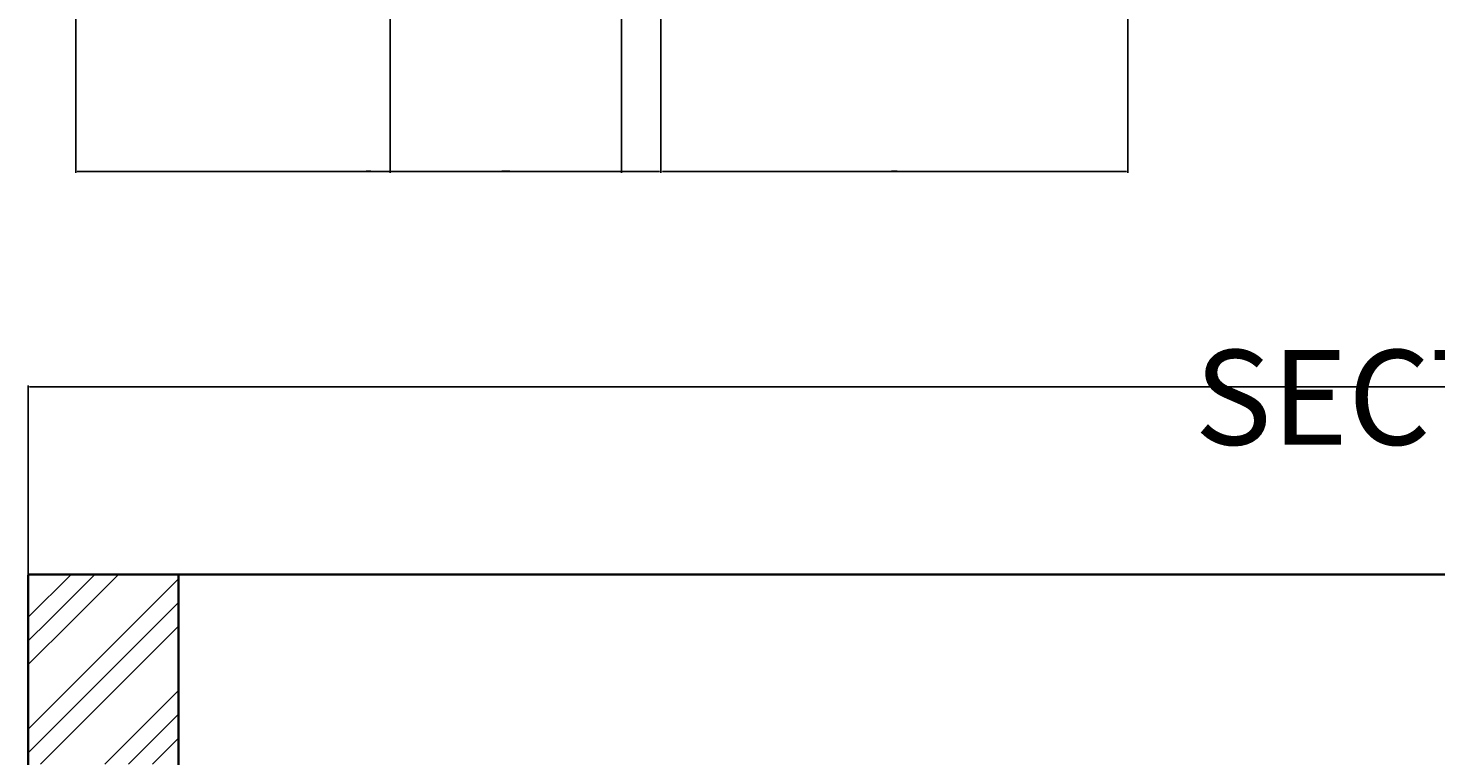
# Model space of a CAD drawing. Units: inches. Extents: x -128 to 854, y -395 to 398.
# Tile 12 of 61: x -56 to 122, y -201 to -109. Entities that reach past the tile are written whole.
import ezdxf

# ---------------------------------------------------------------- set-up
doc = ezdxf.new("R2010")
doc.units = ezdxf.units.IN
doc.header["$MEASUREMENT"] = 0
for name, color, linetype, lineweight in [('A-ANNO-DIMS', 2, 'Continuous', 18), ('A-ANNO-TITL', 7, 'Continuous', 25), ('A-SECT', 220, 'Continuous', 35), ('A-SECT-PATT', 8, 'Continuous', 13)]:
    doc.layers.add(name, color=color, linetype=linetype, lineweight=lineweight)
doc.styles.get("Standard").update_dxf_attribs({"font": 'arial.ttf'})
doc.dimstyles.get("Standard").update_dxf_attribs({"dimtxt": 0.18, "dimasz": 0.18, "dimexe": 0.18, "dimexo": 0.0625, "dimgap": 0.09, "dimtad": 0, "dimtih": 1, "dimtoh": 1, "dimdec": 1, "dimzin": 0, "dimdsep": 46, "dimlunit": 4, "dimtxsty": 'Standard', "dimcen": 0.09, "dimclrd": 1, "dimclre": 2, "dimclrt": 6, "dimadec": 0, "dimazin": 0, "dimtfac": 1, "dimtdec": 1, "dimtofl": 0, "dimtmove": 0, "dimatfit": 3, "dimfxl": 1, "dimtfill": 2, "dimtfillclr": 3, "dimtolj": 1, "dimtzin": 0, "dimarcsym": 0})

# ---------------------------------------------------------------- blocks, each defined once
blk = doc.blocks.new('*D99')
at = {"layer": 'A-ANNO-DIMS', "color": 2, "lineweight": -2, "transparency": 16777216}
for p, q in [((23.85, -89.32), (23.85, -127.24)), ((82.9, -89.32), (82.9, -127.24))]:
    blk.add_line(p, q, dxfattribs=at)
at = {"layer": 'A-ANNO-DIMS', "color": 1, "lineweight": -2, "transparency": 16777216}
for p, q in [((24.03, -127.06), (52.97, -127.06)), ((82.72, -127.06), (53.78, -127.06))]:
    blk.add_line(p, q, dxfattribs=at)
at = {"layer": 'A-ANNO-DIMS', "color": 1, "transparency": 16777216}
for points in [[(24.03, -127.03), (24.03, -127.09), (23.85, -127.06)], [(82.72, -127.03), (82.72, -127.09), (82.9, -127.06)]]:
    blk.add_solid(points, dxfattribs=at)
at = {"layer": 'Defpoints', "color": 0, "transparency": 16777216}
for p in [(23.85, -89.26), (82.9, -89.26), (82.9, -127.06)]:
    blk.add_point(p, dxfattribs=at)
at = {"layer": 'A-ANNO-DIMS', "color": 6, "transparency": 16777216, "insert": (53.37, -127.06), "char_height": 0.18, "attachment_point": 5, "bg_fill": 1, "box_fill_scale": 1.25, "bg_fill_color": 3, "bg_fill_transparency": 0}
blk.add_mtext('\\A1;4\'-11"', dxfattribs=at)
blk = doc.blocks.new('*D100')
at = {"layer": 'A-ANNO-DIMS', "color": 2, "lineweight": -2, "transparency": 16777216}
for p, q in [((-50.13, -89.32), (-50.13, -127.24)), ((23.85, -89.32), (23.85, -127.24))]:
    blk.add_line(p, q, dxfattribs=at)
at = {"layer": 'A-ANNO-DIMS', "color": 1, "lineweight": -2, "transparency": 16777216}
for p, q in [((-49.95, -127.06), (-13.47, -127.06)), ((23.67, -127.06), (-12.81, -127.06))]:
    blk.add_line(p, q, dxfattribs=at)
at = {"layer": 'A-ANNO-DIMS', "color": 1, "transparency": 16777216}
for points in [[(-49.95, -127.03), (-49.95, -127.09), (-50.13, -127.06)], [(23.67, -127.03), (23.67, -127.09), (23.85, -127.06)]]:
    blk.add_solid(points, dxfattribs=at)
at = {"layer": 'Defpoints', "color": 0, "transparency": 16777216}
for p in [(-50.13, -89.26), (23.85, -89.26), (23.85, -127.06)]:
    blk.add_point(p, dxfattribs=at)
at = {"layer": 'A-ANNO-DIMS', "color": 6, "transparency": 16777216, "insert": (-13.14, -127.06), "char_height": 0.18, "attachment_point": 5, "bg_fill": 1, "box_fill_scale": 1.25, "bg_fill_color": 3, "bg_fill_transparency": 0}
blk.add_mtext('\\A1;6\'-2"', dxfattribs=at)
blk = doc.blocks.new('*D102')
at = {"layer": 'A-ANNO-DIMS', "color": 2, "lineweight": -2, "transparency": 16777216}
for p, q in [((-10.39, 39.68), (-10.39, -127.24)), ((18.87, 39.68), (18.87, -127.24))]:
    blk.add_line(p, q, dxfattribs=at)
at = {"layer": 'A-ANNO-DIMS', "color": 1, "lineweight": -2, "transparency": 16777216}
for p, q in [((-10.21, -127.06), (3.7, -127.06)), ((18.69, -127.06), (4.78, -127.06))]:
    blk.add_line(p, q, dxfattribs=at)
at = {"layer": 'A-ANNO-DIMS', "color": 1, "transparency": 16777216}
for points in [[(-10.21, -127.03), (-10.21, -127.09), (-10.39, -127.06)], [(18.69, -127.03), (18.69, -127.09), (18.87, -127.06)]]:
    blk.add_solid(points, dxfattribs=at)
at = {"layer": 'Defpoints', "color": 0, "transparency": 16777216}
for p in [(-10.39, 39.74), (18.87, 39.74), (18.87, -127.06)]:
    blk.add_point(p, dxfattribs=at)
at = {"layer": 'A-ANNO-DIMS', "color": 6, "transparency": 16777216, "insert": (4.24, -127.06), "char_height": 0.18, "attachment_point": 5, "bg_fill": 1, "box_fill_scale": 1.25, "bg_fill_color": 3, "bg_fill_transparency": 0}
blk.add_mtext('\\A1;2\'-5 1/2"', dxfattribs=at)
blk = doc.blocks.new('*D119')
at = {"layer": 'A-ANNO-DIMS', "color": 2, "lineweight": -2, "transparency": 16777216}
for p, q in [((-56.16, -177.96), (-56.16, -154.14)), ((317.84, -177.96), (317.84, -154.14))]:
    blk.add_line(p, q, dxfattribs=at)
at = {"layer": 'A-ANNO-DIMS', "color": 1, "lineweight": -2, "transparency": 16777216}
for p, q in [((-55.98, -154.32), (130.44, -154.32)), ((317.66, -154.32), (131.24, -154.32))]:
    blk.add_line(p, q, dxfattribs=at)
at = {"layer": 'A-ANNO-DIMS', "color": 1, "transparency": 16777216}
for points in [[(-55.98, -154.29), (-55.98, -154.35), (-56.16, -154.32)], [(317.66, -154.29), (317.66, -154.35), (317.84, -154.32)]]:
    blk.add_solid(points, dxfattribs=at)
at = {"layer": 'Defpoints', "color": 0, "transparency": 16777216}
for p in [(317.84, -154.32), (-56.16, -178.02), (317.84, -178.02)]:
    blk.add_point(p, dxfattribs=at)
at = {"layer": 'A-ANNO-DIMS', "color": 6, "transparency": 16777216, "insert": (130.84, -154.32), "char_height": 0.18, "attachment_point": 5, "bg_fill": 1, "box_fill_scale": 1.25, "bg_fill_color": 3, "bg_fill_transparency": 0}
blk.add_mtext('\\A1;31\'-2"', dxfattribs=at)

msp = doc.modelspace()

# ---------------------------------------------------------------- hatches: boundary and pattern name
at = {"layer": 'A-SECT-PATT'}
h = msp.add_hatch(dxfattribs=at)
h.set_pattern_fill('GOST_GROUND', color=256)
h.set_pattern_definition([(45, (0, 0), (14.14214, -9e-16), [20]), (45, (3, 0), (14.14214, -9e-16), [20]), (45, (6, 0), (14.14214, -9e-16), [20])])
h.paths.add_polyline_path([(-37.16, -178.02), (-56.16, -178.02), (-56.16, -202.02), (-37.16, -202.02)])
h.paths.add_polyline_path([(160.84, -178.02), (141.84, -178.02), (141.84, -202.02), (160.84, -202.02)])
h.paths.add_polyline_path([(160.84, -207.02), (141.84, -207.02), (141.84, -226.02), (160.84, -226.02)])
h.paths.add_polyline_path([(317.84, -178.02), (298.84, -178.02), (298.84, -202.02), (317.84, -202.02)])
h.paths.add_polyline_path([(317.84, -207.02), (298.84, -207.02), (298.84, -226.02), (317.84, -226.02)])
h.paths.add_polyline_path([(317.84, -274.02), (298.84, -274.02), (298.84, -298.02), (303.84, -298.02), (312.84, -298.02), (317.84, -298.02)])

# ---------------------------------------------------------------- linework, layer by layer
at = {"layer": 'A-SECT'}
for p, q in [((-56.16, -178.02), (317.84, -178.02)), ((-56.16, -298.02), (-56.16, -178.02)), ((-37.16, -298.02), (-37.16, -178.02))]:
    msp.add_line(p, q, dxfattribs=at)

# ---------------------------------------------------------------- texts
at = {"layer": 'A-ANNO-TITL'}
msp.add_text('SECTION', height=12, dxfattribs=at).set_placement((91.33, -161.64))

# ---------------------------------------------------------------- dimensions: what is measured, and where the dimension line sits
at = {"layer": 'A-ANNO-DIMS'}
for base, p1, p2, picture, middle in [((18.87, -127.06), (-10.39, 39.74), (18.87, 39.74), '*D102', (4.24, -127.06)), ((23.85, -127.06), (-50.13, -89.26), (23.85, -89.26), '*D100', (-13.14, -127.06)), ((82.9003, -127.0595), (23.8451, -89.2595), (82.9003, -89.2595), '*D99', (53.3727, -127.0595)), ((317.84, -154.32), (-56.16, -178.02), (317.84, -178.02), '*D119', (130.84, -154.32))]:
    dim = msp.add_linear_dim(base=base, p1=p1, p2=p2, dimstyle='Standard', override={"dimdec": 1, "dimlfac": 1, "dimrnd": 0, "dimzin": 1, "dimdsep": 46, "dimlunit": 4, "dimfrac": 2}, dxfattribs=at)
    dim.commit()
    dim.dimension.update_dxf_attribs({"geometry": picture, "text_midpoint": middle})

doc.saveas('drawing.dxf')
